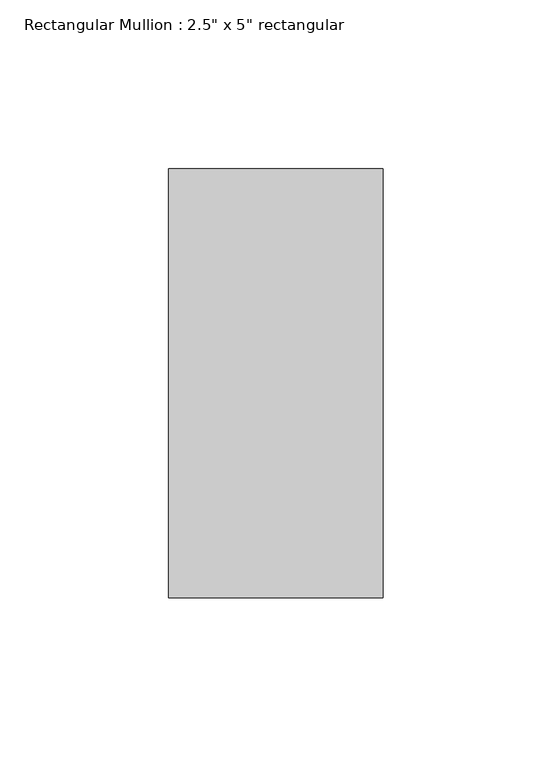
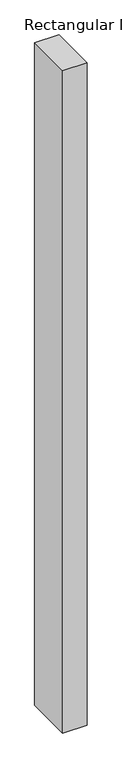
"""IFC4 building model written with IfcOpenShell, lengths in millimetres: member geometry."""

from ifc_helpers import new_model, si_unit, frame, origin, place, context, project, spatial, polyline, outline, extrude, source, transform, mapped, element, save


def member_2fae0574(model_context):
    return source(origin(), model_context, "Body", "SweptSolid", [
        extrude(outline(polyline([(0.0, 63.5), (0.0, -63.5), (-63.5, -63.5), (-63.5, 63.5), (0.0, 63.5)])), frame((0.0, 0.0, -1828.8), z_axis=(0.0, 0.0, 1.0), x_axis=(1.0, 0.0, 0.0)), (0.0, 0.0, 1.0), 1828.8),
    ])


if __name__ == "__main__":
    model = new_model("IFC4")
    model_context = context("Model", 3, world=origin())
    ifc_project = project(units=[si_unit("LENGTHUNIT", "METRE", prefix="MILLI")], contexts=[model_context])
    site = spatial("IfcSite", under=ifc_project)
    building = spatial("IfcBuilding", under=site)
    placement = place(None, origin())
    member_shape = member_2fae0574(model_context)
    element("IfcMember", 1, ObjectType="Rectangular Mullion : 2.5\" x 5\" rectangular", at=placement, inside=building, context=model_context, shape_type="MappedRepresentation", body=[
        mapped(member_shape, transform((0.0, 0.0, 0.0), x_axis=(1.0, 0.0, 0.0), y_axis=(0.0, 1.0, 0.0), z_axis=(0.0, 0.0, 1.0))),
    ])
    save(model, "model.ifc")

# Revit data of these elements
# Type "Rectangular Mullion : 2.5\" x 5\" rectangular"
#   built-in parameter 1007304 = 0.416667 (stored number, unit not read)
#   built-in parameter 1007301 = 0.104167 (stored number, unit not read)
#   built-in parameter 1007300 = 0.104167 (stored number, unit not read)
# Element 1 (IfcMember, "Rectangular Mullion : 2.5\" x 5\" rectangular")
#   Materials on its faces: "Iron, Ductile"
# Materials
#   "Iron, Ductile": class "Metal", colour RGB 0 0 0, transparency 0, Description = "Ductile cast iron", Cost = 0
